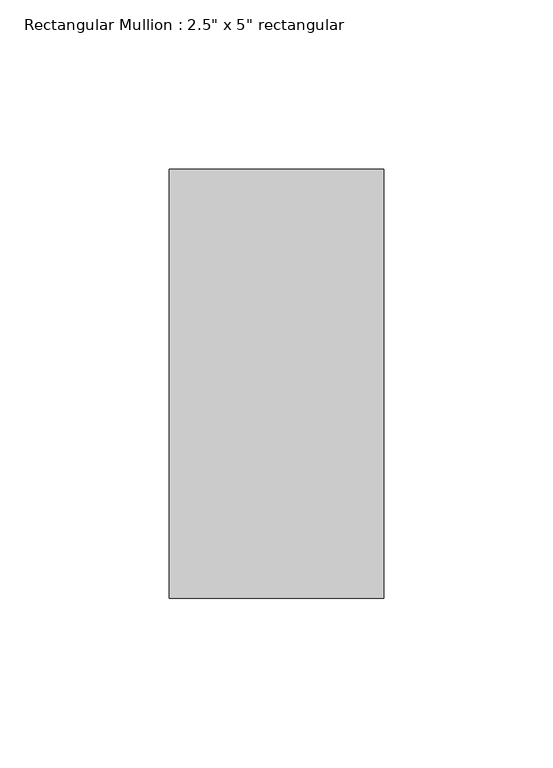
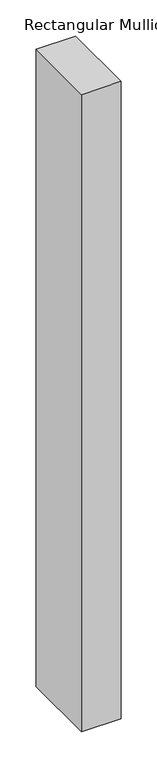
"""IFC4 building model written with IfcOpenShell, lengths in millimetres: member geometry."""

from ifc_helpers import new_model, si_unit, frame, origin, place, context, project, spatial, polyline, outline, extrude, source, transform, mapped, element, save


def member_9c6a9240(model_context):
    return source(origin(), model_context, "Body", "SweptSolid", [
        extrude(outline(polyline([(0.0, 63.5), (0.0, -63.5), (-63.5, -63.5), (-63.5, 63.5), (0.0, 63.5)])), frame((0.0, 0.0, -1079.7501856), z_axis=(0.0, 0.0, 1.0), x_axis=(1.0, 0.0, 0.0)), (0.0, 0.0, 1.0), 1079.7501856),
    ])


if __name__ == "__main__":
    model = new_model("IFC4")
    model_context = context("Model", 3, world=origin())
    ifc_project = project(units=[si_unit("LENGTHUNIT", "METRE", prefix="MILLI")], contexts=[model_context])
    site = spatial("IfcSite", under=ifc_project)
    building = spatial("IfcBuilding", under=site)
    placement = place(None, origin())
    member_shape = member_9c6a9240(model_context)
    element("IfcMember", 1, ObjectType="Rectangular Mullion : 2.5\" x 5\" rectangular", at=placement, inside=building, context=model_context, shape_type="MappedRepresentation", body=[
        mapped(member_shape, transform((0.0, 0.0, 0.0), x_axis=(1.0, 0.0, 0.0), y_axis=(0.0, 1.0, 0.0), z_axis=(0.0, 0.0, 1.0))),
    ])
    save(model, "model.ifc")

# Revit data of these elements
# Type "Rectangular Mullion : 2.5\" x 5\" rectangular"
#   built-in parameter 1007304 = 0.416667 (stored number, unit not read)
#   built-in parameter 1007301 = 0.104167 (stored number, unit not read)
#   built-in parameter 1007300 = 0.104167 (stored number, unit not read)
# Element 1 (IfcMember, "Rectangular Mullion : 2.5\" x 5\" rectangular")
#   Materials on its faces: "Aluminum"
# Materials
#   "Aluminum": class "Metal", colour RGB 247 247 247, transparency 0, Description = "Aluminum 6061", Cost = 0
